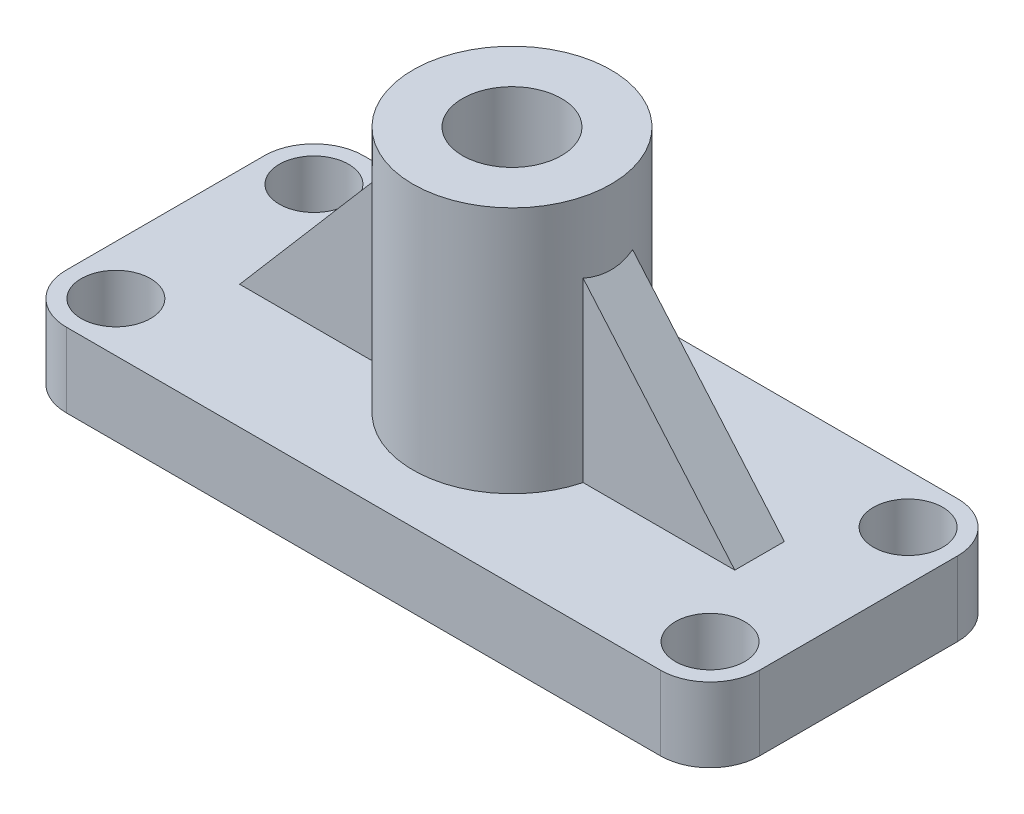
ISO-10303-21;
HEADER;
FILE_DESCRIPTION(('STEP AP214'),'2;1');
FILE_NAME('part.step','',(''),(''),'','','');
FILE_SCHEMA(('AUTOMOTIVE_DESIGN { 1 0 10303 214 1 1 1 1 }'));
ENDSEC;
DATA;
#1=APPLICATION_CONTEXT('core data for automotive mechanical design processes');
#2=APPLICATION_PROTOCOL_DEFINITION('international standard','automotive_design',2000,#1);
#3=PRODUCT_CONTEXT('',#1,'mechanical');
#4=PRODUCT('Part','Part','',(#3));
#5=PRODUCT_RELATED_PRODUCT_CATEGORY('part','',(#4));
#6=PRODUCT_DEFINITION_FORMATION('','',#4);
#7=PRODUCT_DEFINITION_CONTEXT('part definition',#1,'design');
#8=PRODUCT_DEFINITION('design','',#6,#7);
#9=PRODUCT_DEFINITION_SHAPE('','',#8);
#10=(LENGTH_UNIT() NAMED_UNIT(*) SI_UNIT(.MILLI.,.METRE.));
#11=(NAMED_UNIT(*) PLANE_ANGLE_UNIT() SI_UNIT($,.RADIAN.));
#12=(NAMED_UNIT(*) SI_UNIT($,.STERADIAN.) SOLID_ANGLE_UNIT());
#13=UNCERTAINTY_MEASURE_WITH_UNIT(LENGTH_MEASURE(1.E-05),#10,'distance_accuracy_value','');
#14=(GEOMETRIC_REPRESENTATION_CONTEXT(3) GLOBAL_UNCERTAINTY_ASSIGNED_CONTEXT((#13)) GLOBAL_UNIT_ASSIGNED_CONTEXT((#10,
#11,#12)) REPRESENTATION_CONTEXT('',''));
#15=CARTESIAN_POINT('',(0.,0.,0.));
#16=DIRECTION('',(0.,0.,1.));
#17=DIRECTION('',(1.,0.,0.));
#18=AXIS2_PLACEMENT_3D('',#15,#16,#17);
#19=CARTESIAN_POINT('',(70.,15.,0.));
#20=DIRECTION('',(1.,0.,0.));
#21=DIRECTION('',(0.,0.,-1.));
#22=AXIS2_PLACEMENT_3D('',#19,#20,#21);
#23=PLANE('',#22);
#24=DIRECTION('',(0.,-1.,0.));
#25=VECTOR('',#24,1.);
#26=CARTESIAN_POINT('',(70.,15.,20.));
#27=LINE('',#26,#25);
#28=CARTESIAN_POINT('',(70.,15.,20.));
#29=VERTEX_POINT('',#28);
#30=CARTESIAN_POINT('',(70.,0.,20.));
#31=VERTEX_POINT('',#30);
#32=EDGE_CURVE('E243',#29,#31,#27,.T.);
#33=ORIENTED_EDGE('',*,*,#32,.T.);
#34=DIRECTION('',(0.,0.,1.));
#35=VECTOR('',#34,1.);
#36=CARTESIAN_POINT('',(70.,0.,0.));
#37=LINE('',#36,#35);
#38=CARTESIAN_POINT('',(70.,0.,-20.));
#39=VERTEX_POINT('',#38);
#40=EDGE_CURVE('E250',#39,#31,#37,.T.);
#41=ORIENTED_EDGE('',*,*,#40,.F.);
#42=DIRECTION('',(0.,-1.,0.));
#43=VECTOR('',#42,1.);
#44=CARTESIAN_POINT('',(70.,15.,-20.));
#45=LINE('',#44,#43);
#46=CARTESIAN_POINT('',(70.,15.,-20.));
#47=VERTEX_POINT('',#46);
#48=EDGE_CURVE('E11',#47,#39,#45,.T.);
#49=ORIENTED_EDGE('',*,*,#48,.F.);
#50=DIRECTION('',(0.,0.,1.));
#51=VECTOR('',#50,1.);
#52=CARTESIAN_POINT('',(70.,15.,0.));
#53=LINE('',#52,#51);
#54=EDGE_CURVE('E213',#47,#29,#53,.T.);
#55=ORIENTED_EDGE('',*,*,#54,.T.);
#56=EDGE_LOOP('',(#33,#41,#49,#55));
#57=FACE_BOUND('',#56,.T.);
#58=ADVANCED_FACE('F50',(#57),#23,.T.);
#59=CARTESIAN_POINT('',(60.,15.,-20.));
#60=DIRECTION('',(0.,-1.,0.));
#61=DIRECTION('',(0.,0.,-1.));
#62=AXIS2_PLACEMENT_3D('',#59,#60,#61);
#63=CYLINDRICAL_SURFACE('',#62,10.);
#64=CARTESIAN_POINT('',(60.,0.,-20.));
#65=DIRECTION('',(0.,1.,0.));
#66=DIRECTION('',(0.,0.,1.));
#67=AXIS2_PLACEMENT_3D('',#64,#65,#66);
#68=CIRCLE('',#67,10.);
#69=CARTESIAN_POINT('',(60.,0.,-30.));
#70=VERTEX_POINT('',#69);
#71=EDGE_CURVE('E249',#39,#70,#68,.T.);
#72=ORIENTED_EDGE('',*,*,#71,.T.);
#73=DIRECTION('',(0.,-1.,0.));
#74=VECTOR('',#73,1.);
#75=CARTESIAN_POINT('',(60.,15.,-30.));
#76=LINE('',#75,#74);
#77=CARTESIAN_POINT('',(60.,15.,-30.));
#78=VERTEX_POINT('',#77);
#79=EDGE_CURVE('E54',#78,#70,#76,.T.);
#80=ORIENTED_EDGE('',*,*,#79,.F.);
#81=CARTESIAN_POINT('',(60.,15.,-20.));
#82=DIRECTION('',(0.,1.,0.));
#83=DIRECTION('',(0.,0.,1.));
#84=AXIS2_PLACEMENT_3D('',#81,#82,#83);
#85=CIRCLE('',#84,10.);
#86=EDGE_CURVE('E214',#47,#78,#85,.T.);
#87=ORIENTED_EDGE('',*,*,#86,.F.);
#88=ORIENTED_EDGE('',*,*,#48,.T.);
#89=EDGE_LOOP('',(#72,#80,#87,#88));
#90=FACE_BOUND('',#89,.T.);
#91=ADVANCED_FACE('F297',(#90),#63,.T.);
#92=CARTESIAN_POINT('',(0.,15.,-30.));
#93=DIRECTION('',(0.,0.,1.));
#94=DIRECTION('',(1.,0.,0.));
#95=AXIS2_PLACEMENT_3D('',#92,#93,#94);
#96=PLANE('',#95);
#97=DIRECTION('',(-1.,0.,0.));
#98=VECTOR('',#97,1.);
#99=CARTESIAN_POINT('',(0.,0.,-30.));
#100=LINE('',#99,#98);
#101=CARTESIAN_POINT('',(-59.9999999999999,0.,-30.));
#102=VERTEX_POINT('',#101);
#103=EDGE_CURVE('E252',#70,#102,#100,.T.);
#104=ORIENTED_EDGE('',*,*,#103,.T.);
#105=DIRECTION('',(0.,-1.,0.));
#106=VECTOR('',#105,1.);
#107=CARTESIAN_POINT('',(-59.9999999999999,15.,-30.));
#108=LINE('',#107,#106);
#109=CARTESIAN_POINT('',(-59.9999999999999,15.,-30.));
#110=VERTEX_POINT('',#109);
#111=EDGE_CURVE('E288',#110,#102,#108,.T.);
#112=ORIENTED_EDGE('',*,*,#111,.F.);
#113=DIRECTION('',(-1.,0.,0.));
#114=VECTOR('',#113,1.);
#115=CARTESIAN_POINT('',(0.,15.,-30.));
#116=LINE('',#115,#114);
#117=EDGE_CURVE('E217',#78,#110,#116,.T.);
#118=ORIENTED_EDGE('',*,*,#117,.F.);
#119=ORIENTED_EDGE('',*,*,#79,.T.);
#120=EDGE_LOOP('',(#104,#112,#118,#119));
#121=FACE_BOUND('',#120,.T.);
#122=ADVANCED_FACE('F291',(#121),#96,.F.);
#123=CARTESIAN_POINT('',(-60.,15.,-20.));
#124=DIRECTION('',(0.,-1.,0.));
#125=DIRECTION('',(0.,0.,-1.));
#126=AXIS2_PLACEMENT_3D('',#123,#124,#125);
#127=CYLINDRICAL_SURFACE('',#126,10.);
#128=CARTESIAN_POINT('',(-60.,0.,-20.));
#129=DIRECTION('',(0.,1.,0.));
#130=DIRECTION('',(0.,0.,1.));
#131=AXIS2_PLACEMENT_3D('',#128,#129,#130);
#132=CIRCLE('',#131,10.);
#133=CARTESIAN_POINT('',(-70.,0.,-19.9999999999999));
#134=VERTEX_POINT('',#133);
#135=EDGE_CURVE('E254',#102,#134,#132,.T.);
#136=ORIENTED_EDGE('',*,*,#135,.T.);
#137=DIRECTION('',(0.,-1.,0.));
#138=VECTOR('',#137,1.);
#139=CARTESIAN_POINT('',(-70.,15.,-19.9999999999999));
#140=LINE('',#139,#138);
#141=CARTESIAN_POINT('',(-70.,15.,-19.9999999999999));
#142=VERTEX_POINT('',#141);
#143=EDGE_CURVE('E281',#142,#134,#140,.T.);
#144=ORIENTED_EDGE('',*,*,#143,.F.);
#145=CARTESIAN_POINT('',(-60.,15.,-20.));
#146=DIRECTION('',(0.,1.,0.));
#147=DIRECTION('',(0.,0.,1.));
#148=AXIS2_PLACEMENT_3D('',#145,#146,#147);
#149=CIRCLE('',#148,10.);
#150=EDGE_CURVE('E222',#110,#142,#149,.T.);
#151=ORIENTED_EDGE('',*,*,#150,.F.);
#152=ORIENTED_EDGE('',*,*,#111,.T.);
#153=EDGE_LOOP('',(#136,#144,#151,#152));
#154=FACE_BOUND('',#153,.T.);
#155=ADVANCED_FACE('F321',(#154),#127,.T.);
#156=CARTESIAN_POINT('',(-70.,15.,0.));
#157=DIRECTION('',(1.,0.,0.));
#158=DIRECTION('',(0.,0.,-1.));
#159=AXIS2_PLACEMENT_3D('',#156,#157,#158);
#160=PLANE('',#159);
#161=DIRECTION('',(0.,-1.,0.));
#162=VECTOR('',#161,1.);
#163=CARTESIAN_POINT('',(-70.,15.,19.9999999999999));
#164=LINE('',#163,#162);
#165=CARTESIAN_POINT('',(-70.,15.,19.9999999999999));
#166=VERTEX_POINT('',#165);
#167=CARTESIAN_POINT('',(-70.,0.,19.9999999999999));
#168=VERTEX_POINT('',#167);
#169=EDGE_CURVE('E284',#166,#168,#164,.T.);
#170=ORIENTED_EDGE('',*,*,#169,.F.);
#171=DIRECTION('',(0.,0.,1.));
#172=VECTOR('',#171,1.);
#173=CARTESIAN_POINT('',(-70.,15.,0.));
#174=LINE('',#173,#172);
#175=EDGE_CURVE('E221',#142,#166,#174,.T.);
#176=ORIENTED_EDGE('',*,*,#175,.F.);
#177=ORIENTED_EDGE('',*,*,#143,.T.);
#178=DIRECTION('',(0.,0.,1.));
#179=VECTOR('',#178,1.);
#180=CARTESIAN_POINT('',(-70.,0.,0.));
#181=LINE('',#180,#179);
#182=EDGE_CURVE('E256',#134,#168,#181,.T.);
#183=ORIENTED_EDGE('',*,*,#182,.T.);
#184=EDGE_LOOP('',(#170,#176,#177,#183));
#185=FACE_BOUND('',#184,.T.);
#186=ADVANCED_FACE('F318',(#185),#160,.F.);
#187=CARTESIAN_POINT('',(-60.,15.,20.));
#188=DIRECTION('',(0.,-1.,0.));
#189=DIRECTION('',(0.,0.,-1.));
#190=AXIS2_PLACEMENT_3D('',#187,#188,#189);
#191=CYLINDRICAL_SURFACE('',#190,10.);
#192=CARTESIAN_POINT('',(-60.,0.,20.));
#193=DIRECTION('',(0.,1.,0.));
#194=DIRECTION('',(0.,0.,1.));
#195=AXIS2_PLACEMENT_3D('',#192,#193,#194);
#196=CIRCLE('',#195,10.);
#197=CARTESIAN_POINT('',(-59.9999999999999,0.,30.));
#198=VERTEX_POINT('',#197);
#199=EDGE_CURVE('E257',#168,#198,#196,.T.);
#200=ORIENTED_EDGE('',*,*,#199,.T.);
#201=DIRECTION('',(0.,-1.,0.));
#202=VECTOR('',#201,1.);
#203=CARTESIAN_POINT('',(-59.9999999999999,15.,30.));
#204=LINE('',#203,#202);
#205=CARTESIAN_POINT('',(-59.9999999999999,15.,30.));
#206=VERTEX_POINT('',#205);
#207=EDGE_CURVE('E276',#206,#198,#204,.T.);
#208=ORIENTED_EDGE('',*,*,#207,.F.);
#209=CARTESIAN_POINT('',(-60.,15.,20.));
#210=DIRECTION('',(0.,1.,0.));
#211=DIRECTION('',(0.,0.,1.));
#212=AXIS2_PLACEMENT_3D('',#209,#210,#211);
#213=CIRCLE('',#212,10.);
#214=EDGE_CURVE('E228',#166,#206,#213,.T.);
#215=ORIENTED_EDGE('',*,*,#214,.F.);
#216=ORIENTED_EDGE('',*,*,#169,.T.);
#217=EDGE_LOOP('',(#200,#208,#215,#216));
#218=FACE_BOUND('',#217,.T.);
#219=ADVANCED_FACE('F312',(#218),#191,.T.);
#220=CARTESIAN_POINT('',(0.,15.,30.));
#221=DIRECTION('',(0.,0.,-1.));
#222=DIRECTION('',(-1.,0.,0.));
#223=AXIS2_PLACEMENT_3D('',#220,#221,#222);
#224=PLANE('',#223);
#225=DIRECTION('',(1.,0.,0.));
#226=VECTOR('',#225,1.);
#227=CARTESIAN_POINT('',(0.,0.,30.));
#228=LINE('',#227,#226);
#229=CARTESIAN_POINT('',(60.,0.,30.));
#230=VERTEX_POINT('',#229);
#231=EDGE_CURVE('E263',#198,#230,#228,.T.);
#232=ORIENTED_EDGE('',*,*,#231,.T.);
#233=DIRECTION('',(0.,-1.,0.));
#234=VECTOR('',#233,1.);
#235=CARTESIAN_POINT('',(60.,15.,30.));
#236=LINE('',#235,#234);
#237=CARTESIAN_POINT('',(60.,15.,30.));
#238=VERTEX_POINT('',#237);
#239=EDGE_CURVE('E277',#238,#230,#236,.T.);
#240=ORIENTED_EDGE('',*,*,#239,.F.);
#241=DIRECTION('',(1.,0.,0.));
#242=VECTOR('',#241,1.);
#243=CARTESIAN_POINT('',(0.,15.,30.));
#244=LINE('',#243,#242);
#245=EDGE_CURVE('E230',#206,#238,#244,.T.);
#246=ORIENTED_EDGE('',*,*,#245,.F.);
#247=ORIENTED_EDGE('',*,*,#207,.T.);
#248=EDGE_LOOP('',(#232,#240,#246,#247));
#249=FACE_BOUND('',#248,.T.);
#250=ADVANCED_FACE('F315',(#249),#224,.F.);
#251=CARTESIAN_POINT('',(60.,15.,-20.));
#252=DIRECTION('',(0.,-1.,0.));
#253=DIRECTION('',(0.,0.,-1.));
#254=AXIS2_PLACEMENT_3D('',#251,#252,#253);
#255=CYLINDRICAL_SURFACE('',#254,6.99999999999998);
#256=CARTESIAN_POINT('',(60.,15.,-20.));
#257=DIRECTION('',(0.,1.,0.));
#258=DIRECTION('',(0.,0.,1.));
#259=AXIS2_PLACEMENT_3D('',#256,#257,#258);
#260=CIRCLE('',#259,6.99999999999998);
#261=CARTESIAN_POINT('',(60.,15.,-13.));
#262=VERTEX_POINT('',#261);
#263=EDGE_CURVE('E231',#262,#262,#260,.F.);
#264=ORIENTED_EDGE('',*,*,#263,.F.);
#265=EDGE_LOOP('',(#264));
#266=FACE_BOUND('',#265,.T.);
#267=CARTESIAN_POINT('',(60.,0.,-20.));
#268=DIRECTION('',(0.,1.,0.));
#269=DIRECTION('',(0.,0.,1.));
#270=AXIS2_PLACEMENT_3D('',#267,#268,#269);
#271=CIRCLE('',#270,6.99999999999998);
#272=CARTESIAN_POINT('',(60.,0.,-13.));
#273=VERTEX_POINT('',#272);
#274=EDGE_CURVE('E267',#273,#273,#271,.F.);
#275=ORIENTED_EDGE('',*,*,#274,.T.);
#276=EDGE_LOOP('',(#275));
#277=FACE_BOUND('',#276,.T.);
#278=ADVANCED_FACE('F354',(#266,#277),#255,.F.);
#279=CARTESIAN_POINT('',(60.,15.,20.));
#280=DIRECTION('',(0.,-1.,0.));
#281=DIRECTION('',(0.,0.,-1.));
#282=AXIS2_PLACEMENT_3D('',#279,#280,#281);
#283=CYLINDRICAL_SURFACE('',#282,10.);
#284=CARTESIAN_POINT('',(60.,0.,20.));
#285=DIRECTION('',(0.,1.,0.));
#286=DIRECTION('',(0.,0.,1.));
#287=AXIS2_PLACEMENT_3D('',#284,#285,#286);
#288=CIRCLE('',#287,10.);
#289=EDGE_CURVE('E266',#230,#31,#288,.T.);
#290=ORIENTED_EDGE('',*,*,#289,.T.);
#291=ORIENTED_EDGE('',*,*,#32,.F.);
#292=CARTESIAN_POINT('',(60.,15.,20.));
#293=DIRECTION('',(0.,1.,0.));
#294=DIRECTION('',(0.,0.,1.));
#295=AXIS2_PLACEMENT_3D('',#292,#293,#294);
#296=CIRCLE('',#295,10.);
#297=EDGE_CURVE('E235',#238,#29,#296,.T.);
#298=ORIENTED_EDGE('',*,*,#297,.F.);
#299=ORIENTED_EDGE('',*,*,#239,.T.);
#300=EDGE_LOOP('',(#290,#291,#298,#299));
#301=FACE_BOUND('',#300,.T.);
#302=ADVANCED_FACE('F307',(#301),#283,.T.);
#303=CARTESIAN_POINT('',(-60.,15.,-20.));
#304=DIRECTION('',(0.,-1.,0.));
#305=DIRECTION('',(0.,0.,-1.));
#306=AXIS2_PLACEMENT_3D('',#303,#304,#305);
#307=CYLINDRICAL_SURFACE('',#306,7.);
#308=CARTESIAN_POINT('',(-60.,15.,-20.));
#309=DIRECTION('',(0.,1.,0.));
#310=DIRECTION('',(0.,0.,1.));
#311=AXIS2_PLACEMENT_3D('',#308,#309,#310);
#312=CIRCLE('',#311,7.);
#313=CARTESIAN_POINT('',(-60.,15.,-13.));
#314=VERTEX_POINT('',#313);
#315=EDGE_CURVE('E207',#314,#314,#312,.T.);
#316=ORIENTED_EDGE('',*,*,#315,.T.);
#317=EDGE_LOOP('',(#316));
#318=FACE_BOUND('',#317,.T.);
#319=CARTESIAN_POINT('',(-60.,0.,-20.));
#320=DIRECTION('',(0.,1.,0.));
#321=DIRECTION('',(0.,0.,1.));
#322=AXIS2_PLACEMENT_3D('',#319,#320,#321);
#323=CIRCLE('',#322,7.);
#324=CARTESIAN_POINT('',(-60.,0.,-13.));
#325=VERTEX_POINT('',#324);
#326=EDGE_CURVE('E245',#325,#325,#323,.T.);
#327=ORIENTED_EDGE('',*,*,#326,.F.);
#328=EDGE_LOOP('',(#327));
#329=FACE_BOUND('',#328,.T.);
#330=ADVANCED_FACE('F344',(#318,#329),#307,.F.);
#331=CARTESIAN_POINT('',(60.,15.,20.));
#332=DIRECTION('',(0.,-1.,0.));
#333=DIRECTION('',(0.,0.,-1.));
#334=AXIS2_PLACEMENT_3D('',#331,#332,#333);
#335=CYLINDRICAL_SURFACE('',#334,6.99999999999999);
#336=CARTESIAN_POINT('',(60.,15.,20.));
#337=DIRECTION('',(0.,1.,0.));
#338=DIRECTION('',(0.,0.,1.));
#339=AXIS2_PLACEMENT_3D('',#336,#337,#338);
#340=CIRCLE('',#339,6.99999999999999);
#341=CARTESIAN_POINT('',(60.,15.,27.));
#342=VERTEX_POINT('',#341);
#343=EDGE_CURVE('E206',#342,#342,#340,.T.);
#344=ORIENTED_EDGE('',*,*,#343,.T.);
#345=EDGE_LOOP('',(#344));
#346=FACE_BOUND('',#345,.T.);
#347=CARTESIAN_POINT('',(60.,0.,20.));
#348=DIRECTION('',(0.,1.,0.));
#349=DIRECTION('',(0.,0.,1.));
#350=AXIS2_PLACEMENT_3D('',#347,#348,#349);
#351=CIRCLE('',#350,6.99999999999999);
#352=CARTESIAN_POINT('',(60.,0.,27.));
#353=VERTEX_POINT('',#352);
#354=EDGE_CURVE('E204',#353,#353,#351,.T.);
#355=ORIENTED_EDGE('',*,*,#354,.F.);
#356=EDGE_LOOP('',(#355));
#357=FACE_BOUND('',#356,.T.);
#358=ADVANCED_FACE('F47',(#346,#357),#335,.F.);
#359=CARTESIAN_POINT('',(-60.,15.,20.));
#360=DIRECTION('',(0.,-1.,0.));
#361=DIRECTION('',(0.,0.,-1.));
#362=AXIS2_PLACEMENT_3D('',#359,#360,#361);
#363=CYLINDRICAL_SURFACE('',#362,6.99999999999999);
#364=CARTESIAN_POINT('',(-60.,15.,20.));
#365=DIRECTION('',(0.,1.,0.));
#366=DIRECTION('',(0.,0.,1.));
#367=AXIS2_PLACEMENT_3D('',#364,#365,#366);
#368=CIRCLE('',#367,6.99999999999999);
#369=CARTESIAN_POINT('',(-60.,15.,27.));
#370=VERTEX_POINT('',#369);
#371=EDGE_CURVE('E236',#370,#370,#368,.F.);
#372=ORIENTED_EDGE('',*,*,#371,.F.);
#373=EDGE_LOOP('',(#372));
#374=FACE_BOUND('',#373,.T.);
#375=CARTESIAN_POINT('',(-60.,0.,20.));
#376=DIRECTION('',(0.,1.,0.));
#377=DIRECTION('',(0.,0.,1.));
#378=AXIS2_PLACEMENT_3D('',#375,#376,#377);
#379=CIRCLE('',#378,6.99999999999999);
#380=CARTESIAN_POINT('',(-60.,0.,27.));
#381=VERTEX_POINT('',#380);
#382=EDGE_CURVE('E209',#381,#381,#379,.F.);
#383=ORIENTED_EDGE('',*,*,#382,.T.);
#384=EDGE_LOOP('',(#383));
#385=FACE_BOUND('',#384,.T.);
#386=ADVANCED_FACE('F322',(#374,#385),#363,.F.);
#387=CARTESIAN_POINT('',(0.,15.,0.));
#388=DIRECTION('',(0.,1.,0.));
#389=DIRECTION('',(0.,0.,1.));
#390=AXIS2_PLACEMENT_3D('',#387,#388,#389);
#391=PLANE('',#390);
#392=ORIENTED_EDGE('',*,*,#297,.T.);
#393=ORIENTED_EDGE('',*,*,#54,.F.);
#394=ORIENTED_EDGE('',*,*,#86,.T.);
#395=ORIENTED_EDGE('',*,*,#117,.T.);
#396=ORIENTED_EDGE('',*,*,#150,.T.);
#397=ORIENTED_EDGE('',*,*,#175,.T.);
#398=ORIENTED_EDGE('',*,*,#214,.T.);
#399=ORIENTED_EDGE('',*,*,#245,.T.);
#400=EDGE_LOOP('',(#392,#393,#394,#395,#396,#397,#398,#399));
#401=FACE_BOUND('',#400,.T.);
#402=DIRECTION('',(0.,0.,1.));
#403=VECTOR('',#402,1.);
#404=CARTESIAN_POINT('',(50.,15.,0.));
#405=LINE('',#404,#403);
#406=CARTESIAN_POINT('',(50.,15.,5.));
#407=VERTEX_POINT('',#406);
#408=CARTESIAN_POINT('',(50.,15.,-5.));
#409=VERTEX_POINT('',#408);
#410=EDGE_CURVE('E194',#407,#409,#405,.F.);
#411=ORIENTED_EDGE('',*,*,#410,.F.);
#412=DIRECTION('',(1.,0.,0.));
#413=VECTOR('',#412,1.);
#414=CARTESIAN_POINT('',(0.,15.,5.));
#415=LINE('',#414,#413);
#416=CARTESIAN_POINT('',(19.3649167310371,15.,5.));
#417=VERTEX_POINT('',#416);
#418=EDGE_CURVE('E187',#417,#407,#415,.T.);
#419=ORIENTED_EDGE('',*,*,#418,.F.);
#420=CARTESIAN_POINT('',(0.,15.,0.));
#421=DIRECTION('',(0.,1.,0.));
#422=DIRECTION('',(0.,0.,1.));
#423=AXIS2_PLACEMENT_3D('',#420,#421,#422);
#424=CIRCLE('',#423,20.);
#425=CARTESIAN_POINT('',(-19.3649167310371,15.,5.));
#426=VERTEX_POINT('',#425);
#427=EDGE_CURVE('E154',#426,#417,#424,.T.);
#428=ORIENTED_EDGE('',*,*,#427,.F.);
#429=DIRECTION('',(1.,0.,0.));
#430=VECTOR('',#429,1.);
#431=CARTESIAN_POINT('',(0.,15.,5.));
#432=LINE('',#431,#430);
#433=CARTESIAN_POINT('',(-50.,15.,5.));
#434=VERTEX_POINT('',#433);
#435=EDGE_CURVE('E64',#434,#426,#432,.T.);
#436=ORIENTED_EDGE('',*,*,#435,.F.);
#437=DIRECTION('',(0.,0.,1.));
#438=VECTOR('',#437,1.);
#439=CARTESIAN_POINT('',(-50.,15.,0.));
#440=LINE('',#439,#438);
#441=CARTESIAN_POINT('',(-50.,15.,-5.));
#442=VERTEX_POINT('',#441);
#443=EDGE_CURVE('E67',#442,#434,#440,.T.);
#444=ORIENTED_EDGE('',*,*,#443,.F.);
#445=DIRECTION('',(1.,0.,0.));
#446=VECTOR('',#445,1.);
#447=CARTESIAN_POINT('',(0.,15.,-5.));
#448=LINE('',#447,#446);
#449=CARTESIAN_POINT('',(-19.3649167310371,15.,-5.));
#450=VERTEX_POINT('',#449);
#451=EDGE_CURVE('E160',#442,#450,#448,.T.);
#452=ORIENTED_EDGE('',*,*,#451,.T.);
#453=CARTESIAN_POINT('',(19.3649167310371,15.,-5.));
#454=VERTEX_POINT('',#453);
#455=EDGE_CURVE('E148',#454,#450,#424,.T.);
#456=ORIENTED_EDGE('',*,*,#455,.F.);
#457=DIRECTION('',(1.,0.,0.));
#458=VECTOR('',#457,1.);
#459=CARTESIAN_POINT('',(0.,15.,-5.));
#460=LINE('',#459,#458);
#461=EDGE_CURVE('E184',#454,#409,#460,.T.);
#462=ORIENTED_EDGE('',*,*,#461,.T.);
#463=EDGE_LOOP('',(#411,#419,#428,#436,#444,#452,#456,#462));
#464=FACE_BOUND('',#463,.T.);
#465=ORIENTED_EDGE('',*,*,#343,.F.);
#466=EDGE_LOOP('',(#465));
#467=FACE_BOUND('',#466,.T.);
#468=ORIENTED_EDGE('',*,*,#315,.F.);
#469=EDGE_LOOP('',(#468));
#470=FACE_BOUND('',#469,.T.);
#471=ORIENTED_EDGE('',*,*,#263,.T.);
#472=EDGE_LOOP('',(#471));
#473=FACE_BOUND('',#472,.T.);
#474=ORIENTED_EDGE('',*,*,#371,.T.);
#475=EDGE_LOOP('',(#474));
#476=FACE_BOUND('',#475,.T.);
#477=ADVANCED_FACE('F158',(#401,#464,#467,#470,#473,#476),#391,.T.);
#478=CARTESIAN_POINT('',(0.,0.,0.));
#479=DIRECTION('',(0.,1.,0.));
#480=DIRECTION('',(0.,0.,1.));
#481=AXIS2_PLACEMENT_3D('',#478,#479,#480);
#482=PLANE('',#481);
#483=CARTESIAN_POINT('',(0.,0.,0.));
#484=DIRECTION('',(0.,1.,0.));
#485=DIRECTION('',(0.,0.,1.));
#486=AXIS2_PLACEMENT_3D('',#483,#484,#485);
#487=CIRCLE('',#486,10.);
#488=CARTESIAN_POINT('',(0.,0.,10.));
#489=VERTEX_POINT('',#488);
#490=EDGE_CURVE('E199',#489,#489,#487,.T.);
#491=ORIENTED_EDGE('',*,*,#490,.T.);
#492=EDGE_LOOP('',(#491));
#493=FACE_BOUND('',#492,.T.);
#494=ORIENTED_EDGE('',*,*,#40,.T.);
#495=ORIENTED_EDGE('',*,*,#289,.F.);
#496=ORIENTED_EDGE('',*,*,#231,.F.);
#497=ORIENTED_EDGE('',*,*,#199,.F.);
#498=ORIENTED_EDGE('',*,*,#182,.F.);
#499=ORIENTED_EDGE('',*,*,#135,.F.);
#500=ORIENTED_EDGE('',*,*,#103,.F.);
#501=ORIENTED_EDGE('',*,*,#71,.F.);
#502=EDGE_LOOP('',(#494,#495,#496,#497,#498,#499,#500,#501));
#503=FACE_BOUND('',#502,.T.);
#504=ORIENTED_EDGE('',*,*,#354,.T.);
#505=EDGE_LOOP('',(#504));
#506=FACE_BOUND('',#505,.T.);
#507=ORIENTED_EDGE('',*,*,#326,.T.);
#508=EDGE_LOOP('',(#507));
#509=FACE_BOUND('',#508,.T.);
#510=ORIENTED_EDGE('',*,*,#274,.F.);
#511=EDGE_LOOP('',(#510));
#512=FACE_BOUND('',#511,.T.);
#513=ORIENTED_EDGE('',*,*,#382,.F.);
#514=EDGE_LOOP('',(#513));
#515=FACE_BOUND('',#514,.T.);
#516=ADVANCED_FACE('F302',(#493,#503,#506,#509,#512,#515),#482,.F.);
#517=CARTESIAN_POINT('',(0.,65.,0.));
#518=DIRECTION('',(0.,-1.,0.));
#519=DIRECTION('',(0.,0.,-1.));
#520=AXIS2_PLACEMENT_3D('',#517,#518,#519);
#521=CYLINDRICAL_SURFACE('',#520,20.);
#522=CARTESIAN_POINT('',(0.,65.,0.));
#523=DIRECTION('',(0.,1.,0.));
#524=DIRECTION('',(0.,0.,1.));
#525=AXIS2_PLACEMENT_3D('',#522,#523,#524);
#526=CIRCLE('',#525,20.);
#527=CARTESIAN_POINT('',(0.,65.,20.));
#528=VERTEX_POINT('',#527);
#529=EDGE_CURVE('E152',#528,#528,#526,.T.);
#530=ORIENTED_EDGE('',*,*,#529,.F.);
#531=EDGE_LOOP('',(#530));
#532=FACE_BOUND('',#531,.T.);
#533=DIRECTION('',(0.,-1.,0.));
#534=VECTOR('',#533,1.);
#535=CARTESIAN_POINT('',(19.3649167310371,65.,5.));
#536=LINE('',#535,#534);
#537=CARTESIAN_POINT('',(19.3649167310371,50.7409304804567,5.));
#538=VERTEX_POINT('',#537);
#539=EDGE_CURVE('E188',#417,#538,#536,.F.);
#540=ORIENTED_EDGE('',*,*,#539,.T.);
#541=CARTESIAN_POINT('',(0.,73.3333333333333,0.));
#542=DIRECTION('',(-0.759256602365297,-0.650791373455969,0.));
#543=DIRECTION('',(0.650791373455969,-0.759256602365297,0.));
#544=AXIS2_PLACEMENT_3D('',#541,#542,#543);
#545=ELLIPSE('',#544,30.731814857643,20.);
#546=CARTESIAN_POINT('',(19.3649167310371,50.7409304804567,-5.));
#547=VERTEX_POINT('',#546);
#548=EDGE_CURVE('E192',#538,#547,#545,.F.);
#549=ORIENTED_EDGE('',*,*,#548,.T.);
#550=DIRECTION('',(0.,-1.,0.));
#551=VECTOR('',#550,1.);
#552=CARTESIAN_POINT('',(19.3649167310371,65.,-5.));
#553=LINE('',#552,#551);
#554=EDGE_CURVE('E155',#454,#547,#553,.F.);
#555=ORIENTED_EDGE('',*,*,#554,.F.);
#556=ORIENTED_EDGE('',*,*,#455,.T.);
#557=DIRECTION('',(0.,-1.,0.));
#558=VECTOR('',#557,1.);
#559=CARTESIAN_POINT('',(-19.3649167310371,65.,-5.));
#560=LINE('',#559,#558);
#561=CARTESIAN_POINT('',(-19.3649167310371,50.7409304804567,-5.));
#562=VERTEX_POINT('',#561);
#563=EDGE_CURVE('E149',#562,#450,#560,.T.);
#564=ORIENTED_EDGE('',*,*,#563,.F.);
#565=CARTESIAN_POINT('',(0.,73.3333333333333,0.));
#566=DIRECTION('',(-0.759256602365297,0.650791373455969,0.));
#567=DIRECTION('',(-0.650791373455969,-0.759256602365297,0.));
#568=AXIS2_PLACEMENT_3D('',#565,#566,#567);
#569=ELLIPSE('',#568,30.731814857643,20.);
#570=CARTESIAN_POINT('',(-19.3649167310371,50.7409304804567,5.));
#571=VERTEX_POINT('',#570);
#572=EDGE_CURVE('E175',#562,#571,#569,.T.);
#573=ORIENTED_EDGE('',*,*,#572,.T.);
#574=DIRECTION('',(0.,-1.,0.));
#575=VECTOR('',#574,1.);
#576=CARTESIAN_POINT('',(-19.3649167310371,65.,5.));
#577=LINE('',#576,#575);
#578=EDGE_CURVE('E162',#571,#426,#577,.T.);
#579=ORIENTED_EDGE('',*,*,#578,.T.);
#580=ORIENTED_EDGE('',*,*,#427,.T.);
#581=EDGE_LOOP('',(#540,#549,#555,#556,#564,#573,#579,#580));
#582=FACE_BOUND('',#581,.T.);
#583=ADVANCED_FACE('F150',(#532,#582),#521,.T.);
#584=CARTESIAN_POINT('',(0.,65.,0.));
#585=DIRECTION('',(0.,1.,0.));
#586=DIRECTION('',(0.,0.,1.));
#587=AXIS2_PLACEMENT_3D('',#584,#585,#586);
#588=PLANE('',#587);
#589=ORIENTED_EDGE('',*,*,#529,.T.);
#590=EDGE_LOOP('',(#589));
#591=FACE_BOUND('',#590,.T.);
#592=CARTESIAN_POINT('',(0.,65.,0.));
#593=DIRECTION('',(0.,1.,0.));
#594=DIRECTION('',(0.,0.,1.));
#595=AXIS2_PLACEMENT_3D('',#592,#593,#594);
#596=CIRCLE('',#595,10.);
#597=CARTESIAN_POINT('',(0.,65.,10.));
#598=VERTEX_POINT('',#597);
#599=EDGE_CURVE('E197',#598,#598,#596,.T.);
#600=ORIENTED_EDGE('',*,*,#599,.F.);
#601=EDGE_LOOP('',(#600));
#602=FACE_BOUND('',#601,.T.);
#603=ADVANCED_FACE('F447',(#591,#602),#588,.T.);
#604=CARTESIAN_POINT('',(0.,-178.,0.));
#605=DIRECTION('',(0.,1.,0.));
#606=DIRECTION('',(0.,0.,1.));
#607=AXIS2_PLACEMENT_3D('',#604,#605,#606);
#608=CYLINDRICAL_SURFACE('',#607,10.);
#609=ORIENTED_EDGE('',*,*,#490,.F.);
#610=EDGE_LOOP('',(#609));
#611=FACE_BOUND('',#610,.T.);
#612=ORIENTED_EDGE('',*,*,#599,.T.);
#613=EDGE_LOOP('',(#612));
#614=FACE_BOUND('',#613,.T.);
#615=ADVANCED_FACE('F460',(#611,#614),#608,.F.);
#616=CARTESIAN_POINT('',(20.,50.,0.));
#617=DIRECTION('',(-0.759256602365297,-0.650791373455969,0.));
#618=DIRECTION('',(0.650791373455969,-0.759256602365297,0.));
#619=AXIS2_PLACEMENT_3D('',#616,#617,#618);
#620=PLANE('',#619);
#621=DIRECTION('',(0.650791373455969,-0.759256602365297,0.));
#622=VECTOR('',#621,1.);
#623=CARTESIAN_POINT('',(20.,50.,5.));
#624=LINE('',#623,#622);
#625=EDGE_CURVE('E179',#538,#407,#624,.T.);
#626=ORIENTED_EDGE('',*,*,#625,.T.);
#627=ORIENTED_EDGE('',*,*,#410,.T.);
#628=DIRECTION('',(0.650791373455969,-0.759256602365297,0.));
#629=VECTOR('',#628,1.);
#630=CARTESIAN_POINT('',(20.,50.,-5.));
#631=LINE('',#630,#629);
#632=EDGE_CURVE('E178',#547,#409,#631,.T.);
#633=ORIENTED_EDGE('',*,*,#632,.F.);
#634=ORIENTED_EDGE('',*,*,#548,.F.);
#635=EDGE_LOOP('',(#626,#627,#633,#634));
#636=FACE_BOUND('',#635,.T.);
#637=ADVANCED_FACE('F470',(#636),#620,.F.);
#638=CARTESIAN_POINT('',(0.,32.5,5.));
#639=DIRECTION('',(0.,0.,1.));
#640=DIRECTION('',(1.,0.,0.));
#641=AXIS2_PLACEMENT_3D('',#638,#639,#640);
#642=PLANE('',#641);
#643=ORIENTED_EDGE('',*,*,#539,.F.);
#644=ORIENTED_EDGE('',*,*,#418,.T.);
#645=ORIENTED_EDGE('',*,*,#625,.F.);
#646=EDGE_LOOP('',(#643,#644,#645));
#647=FACE_BOUND('',#646,.T.);
#648=ADVANCED_FACE('F476',(#647),#642,.T.);
#649=CARTESIAN_POINT('',(0.,32.5,-5.));
#650=DIRECTION('',(0.,0.,1.));
#651=DIRECTION('',(1.,0.,0.));
#652=AXIS2_PLACEMENT_3D('',#649,#650,#651);
#653=PLANE('',#652);
#654=ORIENTED_EDGE('',*,*,#461,.F.);
#655=ORIENTED_EDGE('',*,*,#554,.T.);
#656=ORIENTED_EDGE('',*,*,#632,.T.);
#657=EDGE_LOOP('',(#654,#655,#656));
#658=FACE_BOUND('',#657,.T.);
#659=ADVANCED_FACE('F488',(#658),#653,.F.);
#660=CARTESIAN_POINT('',(-20.,50.,0.));
#661=DIRECTION('',(-0.759256602365297,0.650791373455969,0.));
#662=DIRECTION('',(-0.650791373455969,-0.759256602365297,0.));
#663=AXIS2_PLACEMENT_3D('',#660,#661,#662);
#664=PLANE('',#663);
#665=DIRECTION('',(-0.650791373455969,-0.759256602365297,0.));
#666=VECTOR('',#665,1.);
#667=CARTESIAN_POINT('',(-20.,50.,-5.));
#668=LINE('',#667,#666);
#669=EDGE_CURVE('E167',#562,#442,#668,.T.);
#670=ORIENTED_EDGE('',*,*,#669,.T.);
#671=ORIENTED_EDGE('',*,*,#443,.T.);
#672=DIRECTION('',(-0.650791373455969,-0.759256602365297,0.));
#673=VECTOR('',#672,1.);
#674=CARTESIAN_POINT('',(-20.,50.,5.));
#675=LINE('',#674,#673);
#676=EDGE_CURVE('E170',#571,#434,#675,.T.);
#677=ORIENTED_EDGE('',*,*,#676,.F.);
#678=ORIENTED_EDGE('',*,*,#572,.F.);
#679=EDGE_LOOP('',(#670,#671,#677,#678));
#680=FACE_BOUND('',#679,.T.);
#681=ADVANCED_FACE('F500',(#680),#664,.T.);
#682=CARTESIAN_POINT('',(0.,32.5,-5.));
#683=DIRECTION('',(0.,0.,1.));
#684=DIRECTION('',(1.,0.,0.));
#685=AXIS2_PLACEMENT_3D('',#682,#683,#684);
#686=PLANE('',#685);
#687=ORIENTED_EDGE('',*,*,#451,.F.);
#688=ORIENTED_EDGE('',*,*,#669,.F.);
#689=ORIENTED_EDGE('',*,*,#563,.T.);
#690=EDGE_LOOP('',(#687,#688,#689));
#691=FACE_BOUND('',#690,.T.);
#692=ADVANCED_FACE('F164',(#691),#686,.F.);
#693=CARTESIAN_POINT('',(0.,32.5,5.));
#694=DIRECTION('',(0.,0.,1.));
#695=DIRECTION('',(1.,0.,0.));
#696=AXIS2_PLACEMENT_3D('',#693,#694,#695);
#697=PLANE('',#696);
#698=ORIENTED_EDGE('',*,*,#676,.T.);
#699=ORIENTED_EDGE('',*,*,#435,.T.);
#700=ORIENTED_EDGE('',*,*,#578,.F.);
#701=EDGE_LOOP('',(#698,#699,#700));
#702=FACE_BOUND('',#701,.T.);
#703=ADVANCED_FACE('F513',(#702),#697,.T.);
#704=CLOSED_SHELL('',(#58,#91,#122,#155,#186,#219,#250,#278,#302,#330,#358,#386,#477,#516,#583,
#603,#615,#637,#648,#659,#681,#692,#703));
#705=MANIFOLD_SOLID_BREP('B2',#704);
#706=ADVANCED_BREP_SHAPE_REPRESENTATION('',(#18,#705),#14);
#707=SHAPE_DEFINITION_REPRESENTATION(#9,#706);
ENDSEC;
END-ISO-10303-21;
